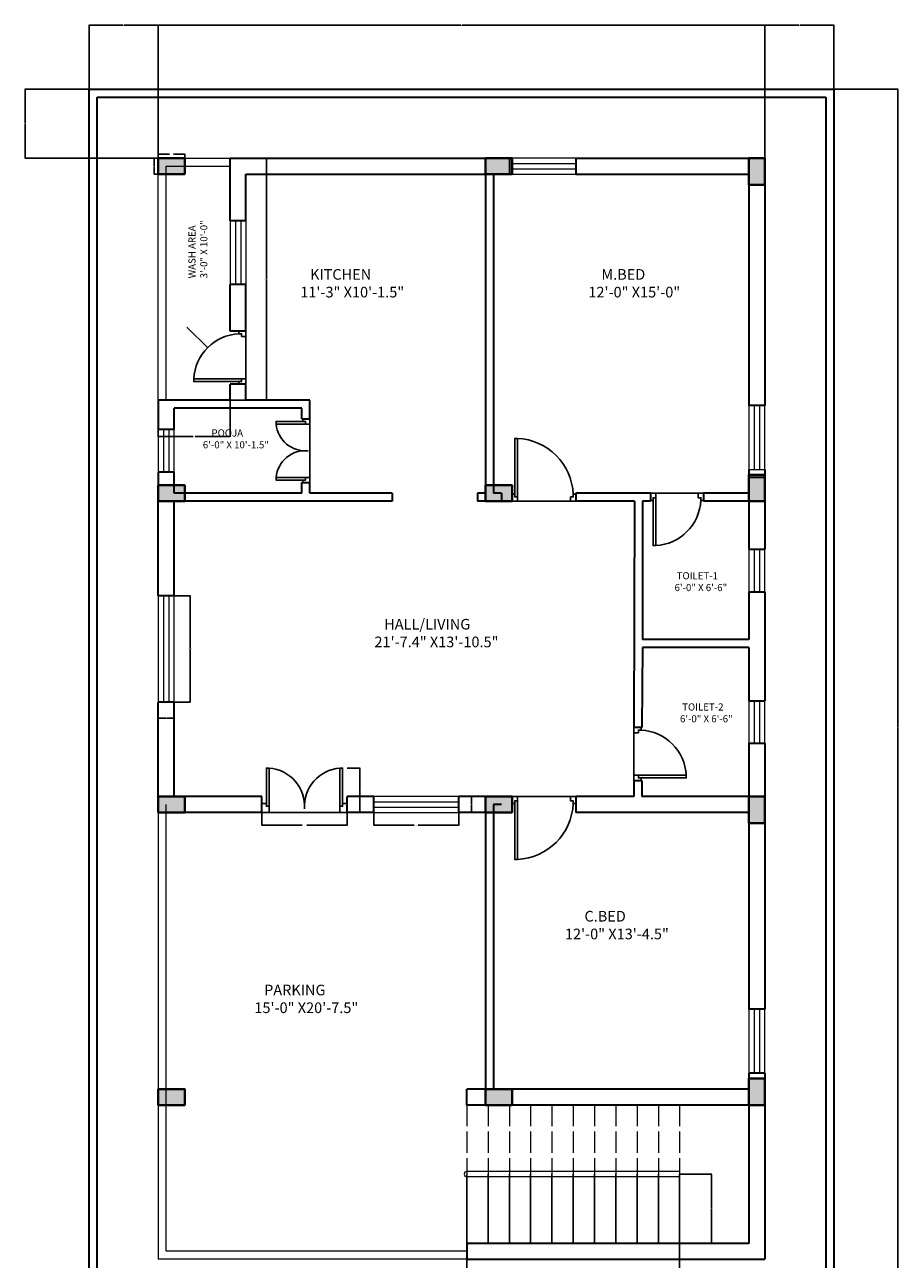
# Model space of a CAD drawing. Units: inches. Extents: x 810 to 2232, y 728 to 1827.
# Tile 2 of 6: x 810 to 1302, y 1131 to 1827. Entities that reach past the tile are written whole.
import ezdxf

# ---------------------------------------------------------------- set-up
doc = ezdxf.new("R2010")
doc.units = ezdxf.units.IN
doc.linetypes.add('ACAD_ISO02W100', pattern=[15, 12, -3])
for name, color, linetype, lineweight in [('A-ANNO-DIMS', 2, 'Continuous', 18), ('A-AREA-IDEN', 50, 'Continuous', 18), ('A-FLOR-STRS-OVHD', 31, 'ACAD_ISO02W100', 18), ('C-SITE-WALL', 7, 'Continuous', 30), ('column', 1, 'Continuous', 40), ('door', 150, 'Continuous', 25), ('railing', 233, 'Continuous', 18), ('staircase', 31, 'Continuous', 25), ('ventilator', 40, 'Continuous', 18), ('Wall', 7, 'Continuous', 35), ('window', 80, 'Continuous', 18)]:
    doc.layers.add(name, color=color, linetype=linetype, lineweight=lineweight)
doc.styles.get("Standard").update_dxf_attribs({"font": 'arial.ttf'})
doc.dimstyles.get("Standard").update_dxf_attribs({"dimtxt": 0.18, "dimasz": 0.18, "dimexe": 0.18, "dimexo": 0.0625, "dimgap": 0.09, "dimtad": 0, "dimtih": 1, "dimtoh": 1, "dimdec": 4, "dimzin": 0, "dimdsep": 46, "dimtxsty": 'Standard', "dimcen": 0.09, "dimadec": 0, "dimazin": 0, "dimtfac": 1, "dimtdec": 4, "dimtofl": 0, "dimtmove": 0, "dimatfit": 3, "dimfxl": 1, "dimtolj": 1, "dimtzin": 0, "dimarcsym": 0})

# ---------------------------------------------------------------- blocks, each defined once
blk = doc.blocks.new('TD')
at = {"layer": 'door'}
blk.add_line((1594.06, 2210.18), (1624.06, 2210.18), dxfattribs=at)
blk.add_lwpolyline([(1595.56, 2212.68), (1597.06, 2212.68), (1597.06, 2239.68), (1595.56, 2239.68)], close=True, dxfattribs=at)
for points in [[(1597.06, 2210.18), (1594.06, 2210.18), (1594.06, 2214.18), (1595.56, 2214.18), (1595.56, 2212.68), (1597.06, 2212.68), (1597.06, 2210.18)], [(1621.06, 2210.18), (1624.06, 2210.18), (1624.06, 2214.18), (1622.56, 2214.18), (1622.56, 2212.68), (1621.06, 2212.68), (1621.06, 2210.18)]]:
    blk.add_lwpolyline(points, dxfattribs=at)
blk.add_arc((1595.56, 2212.68), 27.04, 3.17983, 86.82017, dxfattribs=at)
blk = doc.blocks.new('BD')
at = {"layer": 'door'}
blk.add_line((1349.9, 2199.58), (1385.9, 2199.58), dxfattribs=at)
blk.add_lwpolyline([(1351.4, 2202.08), (1352.9, 2202.08), (1352.9, 2235.08), (1351.4, 2235.08)], close=True, dxfattribs=at)
for points in [[(1352.9, 2199.58), (1349.9, 2199.58), (1349.9, 2203.58), (1351.4, 2203.58), (1351.4, 2202.08), (1352.9, 2202.08), (1352.9, 2199.58)], [(1382.9, 2199.58), (1385.9, 2199.58), (1385.9, 2203.58), (1384.4, 2203.58), (1384.4, 2202.08), (1382.9, 2202.08), (1382.9, 2199.58)]]:
    blk.add_lwpolyline(points, dxfattribs=at)
blk.add_arc((1351.4, 2202.08), 33.03, 2.60256, 87.39744, dxfattribs=at)
blk = doc.blocks.new('PD')
at = {"layer": 'door'}
blk.add_line((1661.56, 2210.18), (1697.56, 2210.18), dxfattribs=at)
for points in [[(1663.06, 2212.68), (1664.56, 2212.68), (1664.56, 2229.18), (1663.06, 2229.18)], [(1694.56, 2212.68), (1696.06, 2212.68), (1696.06, 2229.18), (1694.56, 2229.18)]]:
    blk.add_lwpolyline(points, close=True, dxfattribs=at)
for points in [[(1664.56, 2210.18), (1661.56, 2210.18), (1661.56, 2214.18), (1663.06, 2214.18), (1663.06, 2212.68), (1664.56, 2212.68), (1664.56, 2210.18)], [(1694.56, 2210.18), (1697.56, 2210.18), (1697.56, 2214.18), (1696.06, 2214.18), (1696.06, 2212.68), (1694.56, 2212.68), (1694.56, 2210.18)]]:
    blk.add_lwpolyline(points, dxfattribs=at)
for centre, start, end in [((1663.06, 2212.68), 354.80557, 84.80557), ((1696.06, 2212.68), 95.19443, 185.19443)]:
    blk.add_arc(centre, 16.57, start, end, dxfattribs=at)
blk = doc.blocks.new('HW')
at = {"layer": 'window'}
for p, q in [((1851.89, 1931.95), (1887.89, 1931.95)), ((1851.89, 1928.95), (1887.89, 1928.95))]:
    blk.add_line(p, q, dxfattribs=at)
blk.add_lwpolyline([(1851.89, 1925.95), (1887.89, 1925.95), (1887.89, 1934.95), (1851.89, 1934.95)], close=True, dxfattribs=at)
blk = doc.blocks.new('BW')
at = {"layer": 'window'}
blk.add_blockref('HW', (0, 0), dxfattribs=at)
blk = doc.blocks.new('V')
at = {"layer": 'ventilator'}
for p, q in [((1926.2, 1912.67), (1950.2, 1912.67)), ((1926.2, 1909.67), (1950.2, 1909.67))]:
    blk.add_line(p, q, dxfattribs=at)
blk.add_lwpolyline([(1926.2, 1906.67), (1950.2, 1906.67), (1950.2, 1915.67), (1926.2, 1915.67)], close=True, dxfattribs=at)
blk = doc.blocks.new('MD')
at = {"layer": 'door'}
blk.add_line((1463.68, 2204.78), (1511.68, 2204.78), dxfattribs=at)
for points in [[(1466.18, 2208.28), (1467.68, 2208.28), (1467.68, 2229.78), (1466.18, 2229.78)], [(1507.68, 2208.28), (1509.18, 2208.28), (1509.18, 2229.78), (1507.68, 2229.78)]]:
    blk.add_lwpolyline(points, close=True, dxfattribs=at)
for points in [[(1467.68, 2204.78), (1463.68, 2204.78), (1463.68, 2209.78), (1466.18, 2209.78), (1466.18, 2208.28), (1467.68, 2208.28), (1467.68, 2204.78)], [(1507.68, 2204.78), (1511.68, 2204.78), (1511.68, 2209.78), (1509.18, 2209.78), (1509.18, 2208.28), (1507.68, 2208.28), (1507.68, 2204.78)]]:
    blk.add_lwpolyline(points, dxfattribs=at)
for centre, start, end in [((1466.18, 2208.28), 356.00909, 86.00909), ((1509.18, 2208.28), 93.99091, 183.99091)]:
    blk.add_arc(centre, 21.55, start, end, dxfattribs=at)
blk = doc.blocks.new('DW')
at = {"layer": 'window'}
for p, q in [((1929.05, 1943.86), (1977.05, 1943.86)), ((1929.05, 1940.86), (1977.05, 1940.86))]:
    blk.add_line(p, q, dxfattribs=at)
blk.add_lwpolyline([(1929.05, 1937.86), (1977.05, 1937.86), (1977.05, 1946.86), (1929.05, 1946.86)], close=True, dxfattribs=at)
blk = doc.blocks.new('C1')
at = {"layer": 'column'}
h = blk.add_hatch(color=256, dxfattribs=at)
h.dxf.hatch_style = 1
h.paths.add_polyline_path([(431.83, 1717.82), (446.83, 1717.82), (446.83, 1726.82), (431.83, 1726.82)])
blk.add_lwpolyline([(431.83, 1717.82), (446.83, 1717.82), (446.83, 1726.82), (431.83, 1726.82)], close=True, dxfattribs=at)
blk = doc.blocks.new('W1')
at = {"layer": 'window'}
for p, q in [((710.72, 1551.44), (710.72, 1491.44)), ((713.72, 1551.44), (713.72, 1491.44))]:
    blk.add_line(p, q, dxfattribs=at)
blk.add_lwpolyline([(707.72, 1491.44), (716.72, 1491.44), (716.72, 1551.44), (707.72, 1551.44)], close=True, dxfattribs=at)
blk = doc.blocks.new('STAIR-CENTRE-HANDRAIL')
for p, q in [((121.5, 3), (1.5, 3)), ((121.5, 0), (1.5, 0))]:
    blk.add_line(p, q)
blk.add_arc((1.5, 1.5), 1.5, 90, 270)
blk = doc.blocks.new('RAIL-WASH-RETURN')
for p, q in [((0, 136.5), (40.5, 136.5)), ((0, 0), (0, 136.5)), ((4.5, 0), (4.5, 132)), ((4.5, 132), (40.5, 132))]:
    blk.add_line(p, q)
blk = doc.blocks.new('STAIR-FLIGHT-39IN')
for p, q in [((0, 39), (0, 0)), ((12, 39), (12, 0)), ((24, 39), (24, 0)), ((36, 39), (36, 0)), ((48, 39), (48, 0)), ((60, 39), (60, 0)), ((72, 39), (72, 0)), ((84, 39), (84, 0)), ((96, 39), (96, 0)), ((108, 39), (108, 0)), ((120, 39), (120, 0))]:
    blk.add_line(p, q)
blk = doc.blocks.new('STAIR-FLIGHT-39IN-OVERHEAD')
for p, q in [((0, 39), (0, 0)), ((12, 39), (12, 0)), ((24, 39), (24, 0)), ((36, 39), (36, 0)), ((48, 39), (48, 0)), ((60, 39), (60, 0)), ((72, 39), (72, 0)), ((84, 39), (84, 0)), ((96, 39), (96, 0)), ((108, 39), (108, 0)), ((120, 39), (120, 0))]:
    blk.add_line(p, q)
blk = doc.blocks.new('*D21')
at = {"layer": 'A-ANNO-DIMS', "color": 0, "lineweight": -2, "transparency": 16777216}
for p, q in [((884.83, 1752.01), (884.83, 1754.37)), ((885.01, 1754.19), (891.23, 1754.19)), ((899.65, 1754.19), (893.44, 1754.19)), ((899.83, 1752.01), (899.83, 1754.37))]:
    blk.add_line(p, q, dxfattribs=at)
at = {"layer": 'A-ANNO-DIMS', "color": 0, "transparency": 16777216}
for points in [[(885.01, 1754.22), (885.01, 1754.16), (884.83, 1754.19)], [(899.65, 1754.22), (899.65, 1754.16), (899.83, 1754.19)]]:
    blk.add_solid(points, dxfattribs=at)
at = {"layer": 'Defpoints', "color": 0, "transparency": 16777216}
for p in [(884.83, 1751.94), (899.83, 1754.19), (899.83, 1751.94)]:
    blk.add_point(p, dxfattribs=at)
at = {"layer": 'A-ANNO-DIMS', "color": 0, "transparency": 16777216, "insert": (892.33, 1754.19), "char_height": 0.18, "attachment_point": 5}
blk.add_mtext('\\A1;COLUMN 15 TYP.', dxfattribs=at)
blk = doc.blocks.new('*D22')
at = {"layer": 'A-ANNO-DIMS', "color": 0, "lineweight": -2, "transparency": 16777216}
for p, q in [((884.77, 1751.94), (882.4, 1751.94)), ((882.58, 1751.76), (882.58, 1747.62)), ((884.77, 1742.94), (882.4, 1742.94)), ((882.58, 1743.12), (882.58, 1747.26))]:
    blk.add_line(p, q, dxfattribs=at)
at = {"layer": 'A-ANNO-DIMS', "color": 0, "transparency": 16777216}
for points in [[(882.55, 1751.76), (882.61, 1751.76), (882.58, 1751.94)], [(882.55, 1743.12), (882.61, 1743.12), (882.58, 1742.94)]]:
    blk.add_solid(points, dxfattribs=at)
at = {"layer": 'Defpoints', "color": 0, "transparency": 16777216}
for p in [(882.58, 1751.94), (884.83, 1751.94), (884.83, 1742.94)]:
    blk.add_point(p, dxfattribs=at)
at = {"layer": 'A-ANNO-DIMS', "color": 0, "transparency": 16777216, "insert": (882.58, 1747.44), "char_height": 0.18, "attachment_point": 5}
blk.add_mtext('\\A1;9 TYP.', dxfattribs=at)
blk = doc.blocks.new('*D33')
at = {"layer": 'A-ANNO-DIMS', "color": 0, "lineweight": -2, "transparency": 16777216}
for p, q in [((943.33, 1382.88), (943.33, 1375.56)), ((991.33, 1382.88), (991.33, 1375.56)), ((943.51, 1375.74), (965.94, 1375.74)), ((991.15, 1375.74), (968.73, 1375.74))]:
    blk.add_line(p, q, dxfattribs=at)
at = {"layer": 'A-ANNO-DIMS', "color": 0, "transparency": 16777216}
for points in [[(943.51, 1375.77), (943.51, 1375.71), (943.33, 1375.74)], [(991.15, 1375.77), (991.15, 1375.71), (991.33, 1375.74)]]:
    blk.add_solid(points, dxfattribs=at)
at = {"layer": 'Defpoints', "color": 0, "transparency": 16777216}
for p in [(943.33, 1382.94), (991.33, 1382.94), (991.33, 1375.74)]:
    blk.add_point(p, dxfattribs=at)
at = {"layer": 'A-ANNO-DIMS', "color": 0, "transparency": 16777216, "insert": (967.33, 1375.74), "char_height": 0.18, "attachment_point": 5}
blk.add_mtext('\\A1;ENTRY DOOR 48 TYP.', dxfattribs=at)
blk = doc.blocks.new('*D34')
at = {"layer": 'A-ANNO-DIMS', "color": 0, "lineweight": -2, "transparency": 16777216}
for p, q in [((991.4, 1407.94), (998.71, 1407.94)), ((998.53, 1407.76), (998.53, 1395.62)), ((998.53, 1383.12), (998.53, 1395.26)), ((991.4, 1382.94), (998.71, 1382.94))]:
    blk.add_line(p, q, dxfattribs=at)
at = {"layer": 'A-ANNO-DIMS', "color": 0, "transparency": 16777216}
for points in [[(998.5, 1407.76), (998.56, 1407.76), (998.53, 1407.94)], [(998.5, 1383.12), (998.56, 1383.12), (998.53, 1382.94)]]:
    blk.add_solid(points, dxfattribs=at)
at = {"layer": 'Defpoints', "color": 0, "transparency": 16777216}
for p in [(991.33, 1407.94), (998.53, 1407.94), (991.33, 1382.94)]:
    blk.add_point(p, dxfattribs=at)
at = {"layer": 'A-ANNO-DIMS', "color": 0, "transparency": 16777216, "insert": (998.53, 1395.44), "char_height": 0.18, "attachment_point": 5}
blk.add_mtext('\\A1;25 TYP.', dxfattribs=at)
blk = doc.blocks.new('*D35')
at = {"layer": 'A-ANNO-DIMS', "color": 0, "lineweight": -2, "transparency": 16777216}
for p, q in [((1006.33, 1382.88), (1006.33, 1375.56)), ((1054.33, 1382.88), (1054.33, 1375.56)), ((1006.51, 1375.74), (1029.22, 1375.74)), ((1054.15, 1375.74), (1031.45, 1375.74))]:
    blk.add_line(p, q, dxfattribs=at)
at = {"layer": 'A-ANNO-DIMS', "color": 0, "transparency": 16777216}
for points in [[(1006.51, 1375.77), (1006.51, 1375.71), (1006.33, 1375.74)], [(1054.15, 1375.77), (1054.15, 1375.71), (1054.33, 1375.74)]]:
    blk.add_solid(points, dxfattribs=at)
at = {"layer": 'Defpoints', "color": 0, "transparency": 16777216}
for p in [(1006.33, 1382.94), (1054.33, 1382.94), (1054.33, 1375.74)]:
    blk.add_point(p, dxfattribs=at)
at = {"layer": 'A-ANNO-DIMS', "color": 0, "transparency": 16777216, "insert": (1030.33, 1375.74), "char_height": 0.18, "attachment_point": 5}
blk.add_mtext('\\A1;WINDOW 48 TYP.', dxfattribs=at)
blk = doc.blocks.new('*D36')
at = {"layer": 'A-ANNO-DIMS', "color": 0, "lineweight": -2, "transparency": 16777216}
for p, q in [((1054.4, 1391.94), (1061.71, 1391.94)), ((1061.53, 1391.76), (1061.53, 1387.62)), ((1061.53, 1383.12), (1061.53, 1387.26)), ((1054.4, 1382.94), (1061.71, 1382.94))]:
    blk.add_line(p, q, dxfattribs=at)
at = {"layer": 'A-ANNO-DIMS', "color": 0, "transparency": 16777216}
for points in [[(1061.5, 1391.76), (1061.56, 1391.76), (1061.53, 1391.94)], [(1061.5, 1383.12), (1061.56, 1383.12), (1061.53, 1382.94)]]:
    blk.add_solid(points, dxfattribs=at)
at = {"layer": 'Defpoints', "color": 0, "transparency": 16777216}
for p in [(1054.33, 1391.94), (1061.53, 1391.94), (1054.33, 1382.94)]:
    blk.add_point(p, dxfattribs=at)
at = {"layer": 'A-ANNO-DIMS', "color": 0, "transparency": 16777216, "insert": (1061.53, 1387.44), "char_height": 0.18, "attachment_point": 5}
blk.add_mtext('\\A1;9 TYP.', dxfattribs=at)
blk = doc.blocks.new('*D39')
at = {"layer": 'A-ANNO-DIMS', "color": 0, "lineweight": -2, "transparency": 16777216}
for p, q in [((893.9, 1505.19), (903.01, 1505.19)), ((902.83, 1505.01), (902.83, 1475.38)), ((902.83, 1445.37), (902.83, 1475.01)), ((893.9, 1445.19), (903.01, 1445.19))]:
    blk.add_line(p, q, dxfattribs=at)
at = {"layer": 'A-ANNO-DIMS', "color": 0, "transparency": 16777216}
for points in [[(902.8, 1505.01), (902.86, 1505.01), (902.83, 1505.19)], [(902.8, 1445.37), (902.86, 1445.37), (902.83, 1445.19)]]:
    blk.add_solid(points, dxfattribs=at)
at = {"layer": 'Defpoints', "color": 0, "transparency": 16777216}
for p in [(893.83, 1505.19), (902.83, 1505.19), (893.83, 1445.19)]:
    blk.add_point(p, dxfattribs=at)
at = {"layer": 'A-ANNO-DIMS', "color": 0, "transparency": 16777216, "insert": (902.83, 1475.19), "char_height": 0.18, "attachment_point": 5}
blk.add_mtext('\\A1;HALL WINDOW 60', dxfattribs=at)
blk = doc.blocks.new('*D40')
at = {"layer": 'A-ANNO-DIMS', "color": 0, "lineweight": -2, "transparency": 16777216}
for p, q in [((884.83, 1445.13), (884.83, 1436.01)), ((893.83, 1445.13), (893.83, 1436.01)), ((885.01, 1436.19), (889.18, 1436.19)), ((893.65, 1436.19), (889.48, 1436.19))]:
    blk.add_line(p, q, dxfattribs=at)
at = {"layer": 'A-ANNO-DIMS', "color": 0, "transparency": 16777216}
for points in [[(885.01, 1436.22), (885.01, 1436.16), (884.83, 1436.19)], [(893.65, 1436.22), (893.65, 1436.16), (893.83, 1436.19)]]:
    blk.add_solid(points, dxfattribs=at)
at = {"layer": 'Defpoints', "color": 0, "transparency": 16777216}
for p in [(884.83, 1445.19), (893.83, 1445.19), (893.83, 1436.19)]:
    blk.add_point(p, dxfattribs=at)
at = {"layer": 'A-ANNO-DIMS', "color": 0, "transparency": 16777216, "insert": (889.33, 1436.19), "char_height": 0.18, "attachment_point": 5}
blk.add_mtext('\\A1;9', dxfattribs=at)
blk = doc.blocks.new('*D53')
at = {"layer": 'A-ANNO-DIMS', "color": 0, "lineweight": -2, "transparency": 16777216}
for p, q in [((925.4, 1751.94), (945.99, 1751.94)), ((945.81, 1751.76), (945.81, 1683.88)), ((945.81, 1615.62), (945.81, 1683.51)), ((925.4, 1615.44), (945.99, 1615.44))]:
    blk.add_line(p, q, dxfattribs=at)
at = {"layer": 'A-ANNO-DIMS', "color": 0, "transparency": 16777216}
for points in [[(945.78, 1751.76), (945.84, 1751.76), (945.81, 1751.94)], [(945.78, 1615.62), (945.84, 1615.62), (945.81, 1615.44)]]:
    blk.add_solid(points, dxfattribs=at)
at = {"layer": 'Defpoints', "color": 0, "transparency": 16777216}
for p in [(925.33, 1751.94), (945.81, 1751.94), (925.33, 1615.44)]:
    blk.add_point(p, dxfattribs=at)
at = {"layer": 'A-ANNO-DIMS', "color": 0, "transparency": 16777216, "insert": (945.81, 1683.69), "char_height": 0.18, "attachment_point": 5}
blk.add_mtext('\\A1;WASH RAIL 137 TYP.', dxfattribs=at)
blk = doc.blocks.new('*D54')
at = {"layer": 'A-ANNO-DIMS', "color": 0, "lineweight": -2, "transparency": 16777216}
for p, q in [((884.83, 1615.38), (884.83, 1594.79)), ((925.33, 1615.38), (925.33, 1594.79)), ((885.01, 1594.97), (904.55, 1594.97)), ((925.15, 1594.97), (905.62, 1594.97))]:
    blk.add_line(p, q, dxfattribs=at)
at = {"layer": 'A-ANNO-DIMS', "color": 0, "transparency": 16777216}
for points in [[(885.01, 1595), (885.01, 1594.94), (884.83, 1594.97)], [(925.15, 1595), (925.15, 1594.94), (925.33, 1594.97)]]:
    blk.add_solid(points, dxfattribs=at)
at = {"layer": 'Defpoints', "color": 0, "transparency": 16777216}
for p in [(884.83, 1615.44), (925.33, 1615.44), (925.33, 1594.97)]:
    blk.add_point(p, dxfattribs=at)
at = {"layer": 'A-ANNO-DIMS', "color": 0, "transparency": 16777216, "insert": (905.08, 1594.97), "char_height": 0.18, "attachment_point": 5}
blk.add_mtext('\\A1;41 TYP.', dxfattribs=at)
blk = doc.blocks.new('*D55')
at = {"layer": 'A-ANNO-DIMS', "color": 0, "lineweight": -2, "transparency": 16777216}
for p, q in [((1058.83, 1139.88), (1058.83, 1121.76)), ((1178.83, 1139.88), (1178.83, 1121.76)), ((1059.01, 1121.94), (1117.35, 1121.94)), ((1178.65, 1121.94), (1120.32, 1121.94))]:
    blk.add_line(p, q, dxfattribs=at)
at = {"layer": 'A-ANNO-DIMS', "color": 0, "transparency": 16777216}
for points in [[(1059.01, 1121.97), (1059.01, 1121.91), (1058.83, 1121.94)], [(1178.65, 1121.97), (1178.65, 1121.91), (1178.83, 1121.94)]]:
    blk.add_solid(points, dxfattribs=at)
at = {"layer": 'Defpoints', "color": 0, "transparency": 16777216}
for p in [(1058.83, 1139.94), (1178.83, 1139.94), (1178.83, 1121.94)]:
    blk.add_point(p, dxfattribs=at)
at = {"layer": 'A-ANNO-DIMS', "color": 0, "transparency": 16777216, "insert": (1118.83, 1121.94), "char_height": 0.18, "attachment_point": 5}
blk.add_mtext('\\A1;STAIR FLIGHT 120 TYP.', dxfattribs=at)
blk = doc.blocks.new('*D56')
at = {"layer": 'A-ANNO-DIMS', "color": 0, "lineweight": -2, "transparency": 16777216}
for p, q in [((1178.9, 1178.94), (1197.01, 1178.94)), ((1196.83, 1178.76), (1196.83, 1159.62)), ((1196.83, 1140.12), (1196.83, 1159.26)), ((1178.9, 1139.94), (1197.01, 1139.94))]:
    blk.add_line(p, q, dxfattribs=at)
at = {"layer": 'A-ANNO-DIMS', "color": 0, "transparency": 16777216}
for points in [[(1196.8, 1178.76), (1196.86, 1178.76), (1196.83, 1178.94)], [(1196.8, 1140.12), (1196.86, 1140.12), (1196.83, 1139.94)]]:
    blk.add_solid(points, dxfattribs=at)
at = {"layer": 'Defpoints', "color": 0, "transparency": 16777216}
for p in [(1178.83, 1178.94), (1196.83, 1178.94), (1178.83, 1139.94)]:
    blk.add_point(p, dxfattribs=at)
at = {"layer": 'A-ANNO-DIMS', "color": 0, "transparency": 16777216, "insert": (1196.83, 1159.44), "char_height": 0.18, "attachment_point": 5}
blk.add_mtext('\\A1;39 TYP.', dxfattribs=at)
blk = doc.blocks.new('*D60')
at = {"layer": 'A-ANNO-DIMS', "color": 0, "lineweight": -2, "transparency": 16777216}
for p, q in [((1265.9, 1790.94), (1302.11, 1790.94)), ((1301.93, 1790.76), (1301.93, 1431.12)), ((1301.93, 1071.12), (1301.93, 1430.76)), ((1265.9, 1070.94), (1302.11, 1070.94))]:
    blk.add_line(p, q, dxfattribs=at)
at = {"layer": 'A-ANNO-DIMS', "color": 0, "transparency": 16777216}
for points in [[(1301.9, 1790.76), (1301.96, 1790.76), (1301.93, 1790.94)], [(1301.9, 1071.12), (1301.96, 1071.12), (1301.93, 1070.94)]]:
    blk.add_solid(points, dxfattribs=at)
at = {"layer": 'Defpoints', "color": 0, "transparency": 16777216}
for p in [(1265.83, 1790.94), (1301.93, 1790.94), (1265.83, 1070.94)]:
    blk.add_point(p, dxfattribs=at)
at = {"layer": 'A-ANNO-DIMS', "color": 0, "transparency": 16777216, "insert": (1301.93, 1430.94), "char_height": 0.18, "attachment_point": 5}
blk.add_mtext('\\A1;720', dxfattribs=at)
blk = doc.blocks.new('*D61')
at = {"layer": 'A-ANNO-DIMS', "color": 0, "lineweight": -2, "transparency": 16777216}
for p, q in [((845.83, 1791.01), (845.83, 1827.22)), ((846.01, 1827.04), (865.12, 1827.04)), ((884.65, 1827.04), (865.55, 1827.04)), ((884.83, 1752.01), (884.83, 1827.22))]:
    blk.add_line(p, q, dxfattribs=at)
at = {"layer": 'A-ANNO-DIMS', "color": 0, "transparency": 16777216}
for points in [[(846.01, 1827.07), (846.01, 1827.01), (845.83, 1827.04)], [(884.65, 1827.07), (884.65, 1827.01), (884.83, 1827.04)]]:
    blk.add_solid(points, dxfattribs=at)
at = {"layer": 'Defpoints', "color": 0, "transparency": 16777216}
for p in [(884.83, 1827.04), (845.83, 1790.94), (884.83, 1751.94)]:
    blk.add_point(p, dxfattribs=at)
at = {"layer": 'A-ANNO-DIMS', "color": 0, "transparency": 16777216, "insert": (865.33, 1827.04), "char_height": 0.18, "attachment_point": 5}
blk.add_mtext('\\A1;39', dxfattribs=at)
blk = doc.blocks.new('*D62')
at = {"layer": 'A-ANNO-DIMS', "color": 0, "lineweight": -2, "transparency": 16777216}
for p, q in [((884.83, 1752.01), (884.83, 1827.22)), ((885.01, 1827.04), (1055.55, 1827.04)), ((1226.65, 1827.04), (1056.12, 1827.04)), ((1226.83, 1752.01), (1226.83, 1827.22))]:
    blk.add_line(p, q, dxfattribs=at)
at = {"layer": 'A-ANNO-DIMS', "color": 0, "transparency": 16777216}
for points in [[(885.01, 1827.07), (885.01, 1827.01), (884.83, 1827.04)], [(1226.65, 1827.07), (1226.65, 1827.01), (1226.83, 1827.04)]]:
    blk.add_solid(points, dxfattribs=at)
at = {"layer": 'Defpoints', "color": 0, "transparency": 16777216}
for p in [(1226.83, 1827.04), (884.83, 1751.94), (1226.83, 1751.94)]:
    blk.add_point(p, dxfattribs=at)
at = {"layer": 'A-ANNO-DIMS', "color": 0, "transparency": 16777216, "insert": (1055.83, 1827.04), "char_height": 0.18, "attachment_point": 5}
blk.add_mtext('\\A1;342', dxfattribs=at)
blk = doc.blocks.new('*D63')
at = {"layer": 'A-ANNO-DIMS', "color": 0, "lineweight": -2, "transparency": 16777216}
for p, q in [((1226.83, 1752.01), (1226.83, 1827.22)), ((1227.01, 1827.04), (1246.12, 1827.04)), ((1265.65, 1827.04), (1246.55, 1827.04)), ((1265.83, 1791.01), (1265.83, 1827.22))]:
    blk.add_line(p, q, dxfattribs=at)
at = {"layer": 'A-ANNO-DIMS', "color": 0, "transparency": 16777216}
for points in [[(1227.01, 1827.07), (1227.01, 1827.01), (1226.83, 1827.04)], [(1265.65, 1827.07), (1265.65, 1827.01), (1265.83, 1827.04)]]:
    blk.add_solid(points, dxfattribs=at)
at = {"layer": 'Defpoints', "color": 0, "transparency": 16777216}
for p in [(1265.83, 1827.04), (1265.83, 1790.94), (1226.83, 1751.94)]:
    blk.add_point(p, dxfattribs=at)
at = {"layer": 'A-ANNO-DIMS', "color": 0, "transparency": 16777216, "insert": (1246.33, 1827.04), "char_height": 0.18, "attachment_point": 5}
blk.add_mtext('\\A1;39', dxfattribs=at)
blk = doc.blocks.new('*D65')
at = {"layer": 'A-ANNO-DIMS', "color": 0, "lineweight": -2, "transparency": 16777216}
for p, q in [((845.77, 1790.94), (809.55, 1790.94)), ((809.73, 1790.76), (809.73, 1771.62)), ((809.73, 1752.12), (809.73, 1771.26)), ((884.77, 1751.94), (809.55, 1751.94))]:
    blk.add_line(p, q, dxfattribs=at)
at = {"layer": 'A-ANNO-DIMS', "color": 0, "transparency": 16777216}
for points in [[(809.7, 1790.76), (809.76, 1790.76), (809.73, 1790.94)], [(809.7, 1752.12), (809.76, 1752.12), (809.73, 1751.94)]]:
    blk.add_solid(points, dxfattribs=at)
at = {"layer": 'Defpoints', "color": 0, "transparency": 16777216}
for p in [(809.73, 1790.94), (845.83, 1790.94), (884.83, 1751.94)]:
    blk.add_point(p, dxfattribs=at)
at = {"layer": 'A-ANNO-DIMS', "color": 0, "transparency": 16777216, "insert": (809.73, 1771.44), "char_height": 0.18, "attachment_point": 5}
blk.add_mtext('\\A1;39', dxfattribs=at)
blk = doc.blocks.new('*D94')
at = {"layer": 'A-ANNO-DIMS', "color": 0, "lineweight": -2, "transparency": 16777216}
for p, q in [((901.06, 1656.54), (901.24, 1656.54)), ((901.24, 1656.54), (912.59, 1645.19)), ((931.74, 1625.94), (931.92, 1625.94)), ((931.83, 1625.85), (931.83, 1626.03))]:
    blk.add_line(p, q, dxfattribs=at)
at = {"layer": 'A-ANNO-DIMS', "color": 0, "transparency": 16777216}
blk.add_solid([(912.61, 1645.21), (912.56, 1645.17), (912.71, 1645.06)], dxfattribs=at)
at = {"layer": 'Defpoints', "color": 0, "transparency": 16777216}
for p in [(912.71, 1645.06), (931.83, 1625.94)]:
    blk.add_point(p, dxfattribs=at)
at = {"layer": 'A-ANNO-DIMS', "color": 0, "transparency": 16777216, "insert": (900.39, 1656.54), "char_height": 0.18, "attachment_point": 5}
blk.add_mtext('\\A1;2X R27.04', dxfattribs=at)

msp = doc.modelspace()

# ---------------------------------------------------------------- linework, layer by layer
at = {"layer": 'C-SITE-WALL'}
for p, q in [((845.8341, 1790.9426), (1265.8341, 1790.9426)), ((845.8341, 1070.9426), (845.8341, 1790.9426)), ((1265.8341, 1790.9426), (1265.8341, 1070.9426)), ((850.3341, 1786.4426), (1261.3341, 1786.4426)), ((850.3341, 1079.9426), (850.3341, 1786.4426)), ((1261.3341, 1786.4426), (1261.3341, 1079.9426))]:
    msp.add_line(p, q, dxfattribs=at)
at = {"layer": 'railing'}
for p, q in [((884.8341, 1387.4426), (884.8341, 1130.9426)), ((889.3341, 1135.4426), (889.3341, 1387.4426)), ((1058.8341, 1135.4426), (889.3341, 1135.4426)), ((1058.8341, 1130.9426), (884.8341, 1130.9426))]:
    msp.add_line(p, q, dxfattribs=at)
at = {"layer": 'Wall'}
for p, q in [((925.3341, 1716.6926), (925.3341, 1751.9426)), ((925.3341, 1751.9426), (1082.8341, 1751.9426)), ((1082.8341, 1751.9426), (1082.8341, 1742.9426)), ((1120.3341, 1751.9426), (1226.8341, 1751.9426)), ((1120.3341, 1751.9426), (1120.3341, 1742.9426)), ((1226.8341, 1751.9426), (1226.8341, 1612.4426)), ((934.3341, 1742.9426), (1069.3341, 1742.9426)), ((934.3341, 1716.6926), (934.3341, 1742.9426)), ((1069.3341, 1742.9426), (1069.3341, 1562.9426)), ((1073.8341, 1742.9426), (1082.8341, 1742.9426)), ((1073.8341, 1742.9426), (1073.8341, 1562.9426)), ((1120.3341, 1742.9426), (1217.8341, 1742.9426)), ((1217.8341, 1742.9426), (1217.8341, 1612.4426)), ((934.3341, 1716.6926), (925.3341, 1716.6926)), ((925.3341, 1654.4426), (925.3341, 1680.6926)), ((934.3341, 1680.6926), (925.3341, 1680.6926)), ((934.3341, 1654.4426), (934.3341, 1680.6926)), ((934.3341, 1654.4426), (925.3341, 1654.4426)), ((934.3341, 1624.4426), (925.3341, 1624.4426)), ((925.3341, 1615.4426), (925.3341, 1624.4426)), ((934.3341, 1615.4426), (934.3341, 1624.4426)), ((925.3341, 1615.4426), (884.8341, 1615.4426)), ((884.8341, 1615.4426), (884.8341, 1598.9426)), ((970.3341, 1615.4426), (934.3341, 1615.4426)), ((970.3341, 1604.9426), (970.3341, 1615.4426)), ((965.8341, 1610.9426), (893.8341, 1610.9426)), ((893.8341, 1598.9426), (893.8341, 1610.9426)), ((965.8341, 1604.9426), (965.8341, 1610.9426)), ((1226.8341, 1612.4426), (1217.8341, 1612.4426)), ((965.8341, 1604.9426), (970.3341, 1604.9426)), ((893.8341, 1598.9426), (884.8341, 1598.9426)), ((893.8341, 1574.9426), (884.8341, 1574.9426)), ((884.8341, 1574.9426), (884.8341, 1558.4426)), ((893.8341, 1562.9426), (893.8341, 1574.9426)), ((1217.8341, 1576.4426), (1217.8341, 1531.4426)), ((1226.8341, 1576.4426), (1226.8341, 1531.4426)), ((965.8341, 1562.9426), (965.8341, 1568.9426)), ((965.8341, 1568.9426), (970.3341, 1568.9426)), ((970.3341, 1562.9426), (970.3341, 1568.9426)), ((1217.8341, 1571.9426), (1217.8341, 1562.9426)), ((1226.8341, 1571.9426), (1217.8341, 1571.9426)), ((965.8341, 1562.9426), (893.8341, 1562.9426)), ((1016.8341, 1562.9426), (970.3341, 1562.9426)), ((1016.8341, 1562.9426), (1016.8341, 1558.4426)), ((1064.8341, 1562.9426), (1064.8341, 1558.4426)), ((1069.3341, 1562.9426), (1064.8341, 1562.9426)), ((1078.3341, 1562.9426), (1073.8341, 1562.9426)), ((1078.3341, 1562.9426), (1078.3341, 1558.4426)), ((1120.3341, 1562.9426), (1120.3341, 1558.4426)), ((1162.3341, 1562.9426), (1120.3341, 1562.9426)), ((1162.3341, 1562.9426), (1162.3341, 1558.4426)), ((1192.3341, 1562.9426), (1192.3341, 1558.4426)), ((1217.8341, 1562.9426), (1192.3341, 1562.9426)), ((1016.8341, 1558.4426), (884.8341, 1558.4426)), ((884.8341, 1505.1926), (884.8341, 1558.4426)), ((893.8341, 1505.1926), (893.8341, 1558.4426)), ((1078.3341, 1558.4426), (1064.8341, 1558.4426)), ((1153.3341, 1558.4426), (1120.3341, 1558.4426)), ((1153.3341, 1558.4426), (1153.0841, 1430.9426)), ((1157.8341, 1558.4426), (1157.8341, 1480.4426)), ((1162.3341, 1558.4426), (1157.8341, 1558.4426)), ((1217.8341, 1558.4426), (1192.3341, 1558.4426)), ((1217.8341, 1531.4426), (1226.8341, 1531.4426)), ((893.8341, 1505.1926), (884.8341, 1505.1926)), ((1217.8341, 1507.4426), (1226.8341, 1507.4426)), ((1217.8341, 1507.4426), (1217.8341, 1480.4426)), ((1226.8341, 1507.4426), (1226.8341, 1445.9426)), ((1217.8341, 1480.4426), (1157.8341, 1480.4426)), ((1157.8341, 1475.9426), (1157.5841, 1430.9426)), ((1217.8341, 1475.9426), (1157.8341, 1475.9426)), ((1217.8341, 1475.9426), (1217.8341, 1445.9426)), ((884.8341, 1391.9426), (884.8341, 1445.1926)), ((893.8341, 1445.1926), (884.8341, 1445.1926)), ((893.8341, 1391.9426), (893.8341, 1445.1926)), ((1217.8341, 1445.9426), (1226.8341, 1445.9426)), ((1157.5841, 1430.9426), (1153.0841, 1430.9426)), ((1217.8341, 1421.9426), (1226.8341, 1421.9426)), ((1217.8341, 1421.9426), (1217.8341, 1391.9426)), ((1226.8341, 1421.9426), (1226.8341, 1271.9426)), ((1153.0841, 1400.9426), (1153.0841, 1391.9426)), ((1153.0841, 1400.9426), (1157.5841, 1400.9426)), ((1157.5841, 1400.9426), (1157.5841, 1391.9426)), ((943.3341, 1391.9426), (884.8341, 1391.9426)), ((884.8341, 1391.9426), (884.8341, 1382.9426)), ((943.3341, 1382.9426), (943.3341, 1391.9426)), ((991.3341, 1382.9426), (991.3341, 1391.9426)), ((1006.3341, 1391.9426), (991.3341, 1391.9426)), ((1006.3341, 1382.9426), (1006.3341, 1391.9426)), ((1078.3341, 1391.9426), (1054.3341, 1391.9426)), ((1054.3341, 1382.9426), (1054.3341, 1391.9426)), ((1069.3341, 1387.4426), (1069.3341, 1226.9426)), ((1073.8341, 1387.4426), (1073.8341, 1226.9426)), ((1078.3341, 1387.4426), (1073.8341, 1387.4426)), ((1153.0841, 1391.9426), (1120.3341, 1391.9426)), ((1120.3341, 1391.9426), (1120.3341, 1382.9426)), ((1217.8341, 1391.9426), (1157.5841, 1391.9426)), ((1217.8341, 1387.4426), (1217.8341, 1271.9426)), ((943.3341, 1382.9426), (884.8341, 1382.9426)), ((1006.3341, 1382.9426), (991.3341, 1382.9426)), ((1069.3341, 1382.9426), (1054.3341, 1382.9426)), ((1217.8341, 1382.9426), (1120.3341, 1382.9426)), ((1226.8341, 1271.9426), (1217.8341, 1271.9426)), ((1217.8341, 1235.9426), (1217.8341, 1226.9426)), ((1226.8341, 1235.9426), (1217.8341, 1235.9426)), ((1226.8341, 1235.9426), (1226.8341, 1130.9426)), ((1217.8341, 1226.9426), (1058.8341, 1226.9426)), ((1058.8341, 1217.9426), (1058.8341, 1226.9426)), ((1217.8341, 1217.9426), (1058.8341, 1217.9426)), ((1217.8341, 1217.9426), (1217.8341, 1139.9426)), ((1217.8341, 1139.9426), (1058.8341, 1139.9426)), ((1058.8341, 1139.9426), (1058.8341, 1130.9426)), ((1058.8341, 1130.9426), (1226.8341, 1130.9426))]:
    msp.add_line(p, q, dxfattribs=at)

# ---------------------------------------------------------------- block references
at = {"layer": 'A-FLOR-STRS-OVHD'}
msp.add_blockref('STAIR-FLIGHT-39IN-OVERHEAD', (1058.8341, 1178.9426), dxfattribs=at)
at = {"layer": 'column'}
for p in [(453.0038, 25.1272), (637.5038, 25.1272), (453.0038, -159.3728), (637.5038, -159.3728), (453.0038, -334.8728), (637.5038, -334.8728), (453.0038, -499.8728), (637.5038, -499.8728)]:
    msp.add_blockref('C1', p, dxfattribs=at)
at = {"layer": 'column', "rotation": 90}
for p in [(2944.6494, 1305.1124), (2944.6494, 1126.6124), (2944.6494, 945.1124), (2944.6494, 786.1124)]:
    msp.add_blockref('C1', p, dxfattribs=at)
at = {"layer": 'door', "rotation": 90}
for name, p in [('TD', (3144.5147, 30.3815)), ('PD', (3180.5147, -92.6164))]:
    msp.add_blockref(name, p, dxfattribs=at)
at = {"layer": 'door'}
for name, p in [('BD', (-265.5658, -641.1374)), ('MD', (-520.3508, -821.8359))]:
    msp.add_blockref(name, p, dxfattribs=at)
at = {"layer": 'door', "xscale": -1}
for name, p, rotation in [('TD', (-431.727, 3773.1232), 180), ('TD', (-1057.0966, -193.1185), 270), ('BD', (-265.5658, 3591.5226), 180)]:
    msp.add_blockref(name, p, dxfattribs=dict(at, rotation=rotation))
at = {"layer": 'railing'}
for name, p in [('RAIL-WASH-RETURN', (884.8341, 1615.443)), ('STAIR-CENTRE-HANDRAIL', (1057.3341, 1177.443))]:
    msp.add_blockref(name, p, dxfattribs=at)
at = {"layer": 'staircase'}
msp.add_blockref('STAIR-FLIGHT-39IN', (1058.8341, 1139.9426), dxfattribs=at)
at = {"layer": 'ventilator', "rotation": 270}
for p in [(-1021.834, 3525.1471), (-688.834, 3457.6471), (-688.834, 3372.1471)]:
    msp.add_blockref('V', p, dxfattribs=at)
at = {"layer": 'window'}
for name, p in [('BW', (-767.5574, -183.0026)), ('W1', (177.1126, -46.2427)), ('DW', (-922.7146, -554.9187))]:
    msp.add_blockref(name, p, dxfattribs=at)
at = {"layer": 'window', "rotation": 270}
for p in [(-1000.6112, 3568.5841), (-708.1112, 3464.3341), (-708.1112, 3123.8341)]:
    msp.add_blockref('BW', p, dxfattribs=at)

# ---------------------------------------------------------------- texts
at = {"layer": 'A-AREA-IDEN', "insert": (901.8814, 1684.1833), "char_height": 4, "attachment_point": 1, "rotation": 90}
msp.add_mtext_dynamic_manual_height_columns('WASH AREA \\P3\'-0" X 10\'-0"', width=38.565761, gutter_width=12.5, heights=[0], dxfattribs=at)
at = {"layer": 'A-AREA-IDEN', "attachment_point": 1}
for s, width, insert, char_height in [('   KITCHEN\\P11\'-3" X10\'-1.5" ', 89.482208, (964.9429, 1689.4028), 6), ('    M.BED\\P12\'-0" X15\'-0" ', 89.482208, (1127.383, 1689.4028), 6), ('    POOJA \\P6\'-0" X 10\'-1.5"', 39.097568, (909.9981, 1598.976), 4), (' TOILET-1 \\P6\'-0" X 6\'-6"', 41.756603, (1175.967, 1518.4487), 4), ('   HALL/LIVING\\P21\'-7.4" X13\'-10.5" ', 95.024267, (1006.7527, 1492.1282), 6), (' TOILET-2\\P6\'-0" X 6\'-6"', 41.756609, (1179.053, 1444.4457), 4), ('      C.BED\\P12\'-0" X13\'-4.5" ', 89.482208, (1114.1713, 1327.4241), 6), ('   PARKING\\P15\'-0" X20\'-7.5" ', 105.343087, (939.0587, 1285.8153), 6)]:
    msp.add_mtext_dynamic_manual_height_columns(s, width=width, gutter_width=12.5, heights=[0], dxfattribs=dict(at, insert=insert, char_height=char_height))

# ---------------------------------------------------------------- dimensions: what is measured, and where the dimension line sits
at = {"layer": 'A-ANNO-DIMS'}
for base, p1, p2, picture, middle in [((884.8341, 1827.0426), (845.8341, 1790.9426), (884.8341, 1751.9426), '*D61', (865.3341, 1827.0426)), ((1226.8341, 1827.0426), (884.8341, 1751.9426), (1226.8341, 1751.9426), '*D62', (1055.8341, 1827.0426)), ((1265.8341, 1827.0426), (1226.8341, 1751.9426), (1265.8341, 1790.9426), '*D63', (1246.3341, 1827.0426)), ((893.8341, 1436.1926), (884.8341, 1445.1926), (893.8341, 1445.1926), '*D40', (889.3341, 1436.1926))]:
    dim = msp.add_linear_dim(base=base, p1=p1, p2=p2, dimstyle='Standard', override={"dimdec": 0, "dimlfac": 1, "dimrnd": 0, "dimzin": 0, "dimdsep": 46, "dimlunit": 2}, dxfattribs=at)
    dim.commit()
    dim.dimension.update_dxf_attribs({"geometry": picture, "text_midpoint": middle})
for base, p1, p2, picture, middle in [((809.7341, 1790.9426), (884.8341, 1751.9426), (845.8341, 1790.9426), '*D65', (809.7341, 1771.4426)), ((1301.9341, 1790.9426), (1265.8341, 1070.9426), (1265.8341, 1790.9426), '*D60', (1301.9341, 1430.9426))]:
    dim = msp.add_linear_dim(base=base, p1=p1, p2=p2, angle=90, dimstyle='Standard', override={"dimdec": 0, "dimlfac": 1, "dimrnd": 0, "dimzin": 0, "dimdsep": 46, "dimlunit": 2}, dxfattribs=at)
    dim.commit()
    dim.dimension.update_dxf_attribs({"geometry": picture, "text_midpoint": middle})
for base, p1, p2, text, picture, middle in [((882.5841, 1751.9426), (884.8341, 1742.9426), (884.8341, 1751.9426), '<> TYP.', '*D22', (882.5841, 1747.4426)), ((945.8090622384, 1751.9426203011), (925.3340622384, 1615.4426203011), (925.3340622384, 1751.9426203011), 'WASH RAIL <> TYP.', '*D53', (945.8090622384, 1683.6926203011)), ((902.8341, 1505.1926), (893.8341, 1445.1926), (893.8341, 1505.1926), 'HALL WINDOW <>', '*D39', (902.8341, 1475.1926)), ((998.5341, 1407.9426), (991.3341, 1382.9426), (991.3341, 1407.9426), '<> TYP.', '*D34', (998.5341, 1395.4426)), ((1061.5341, 1391.9426), (1054.3341, 1382.9426), (1054.3341, 1391.9426), '<> TYP.', '*D36', (1061.5341, 1387.4426)), ((1196.8341, 1178.9426), (1178.8341, 1139.9426), (1178.8341, 1178.9426), '<> TYP.', '*D56', (1196.8341, 1159.4426))]:
    dim = msp.add_linear_dim(base=base, p1=p1, p2=p2, angle=90, text=text, dimstyle='Standard', override={"dimdec": 0, "dimlfac": 1, "dimrnd": 0, "dimzin": 0, "dimdsep": 46, "dimlunit": 2}, dxfattribs=at)
    dim.commit()
    dim.dimension.update_dxf_attribs({"geometry": picture, "text_midpoint": middle})
for base, p1, p2, text, picture, middle in [((899.8341, 1754.1926), (884.8341, 1751.9426), (899.8341, 1751.9426), 'COLUMN <> TYP.', '*D21', (892.3341, 1754.1926)), ((925.3340622384, 1594.9676203011), (884.8340622384, 1615.4426203011), (925.3340622384, 1615.4426203011), '<> TYP.', '*D54', (905.0840622384, 1594.9676203011)), ((991.3341, 1375.7426), (943.3341, 1382.9426), (991.3341, 1382.9426), 'ENTRY DOOR <> TYP.', '*D33', (967.3341, 1375.7426)), ((1054.3341, 1375.7426), (1006.3341, 1382.9426), (1054.3341, 1382.9426), 'WINDOW <> TYP.', '*D35', (1030.3341, 1375.7426)), ((1178.8341, 1121.9426), (1058.8341, 1139.9426), (1178.8341, 1139.9426), 'STAIR FLIGHT <> TYP.', '*D55', (1118.8341, 1121.9426))]:
    dim = msp.add_linear_dim(base=base, p1=p1, p2=p2, text=text, dimstyle='Standard', override={"dimdec": 0, "dimlfac": 1, "dimrnd": 0, "dimzin": 0, "dimdsep": 46, "dimlunit": 2}, dxfattribs=at)
    dim.commit()
    dim.dimension.update_dxf_attribs({"geometry": picture, "text_midpoint": middle})
dim = msp.add_radius_dim(center=(931.8341, 1625.9426), mpoint=(912.7129, 1645.0641), text='2X <>', dimstyle='Standard', override={"dimdec": 2, "dimlfac": 1, "dimrnd": 0, "dimzin": 0, "dimdsep": 46, "dimlunit": 2}, dxfattribs=at)
dim.commit()
dim.dimension.update_dxf_attribs({"geometry": '*D94', "text_midpoint": (900.3858, 1656.537), "dimtype": 164})

doc.saveas('drawing.dxf')
